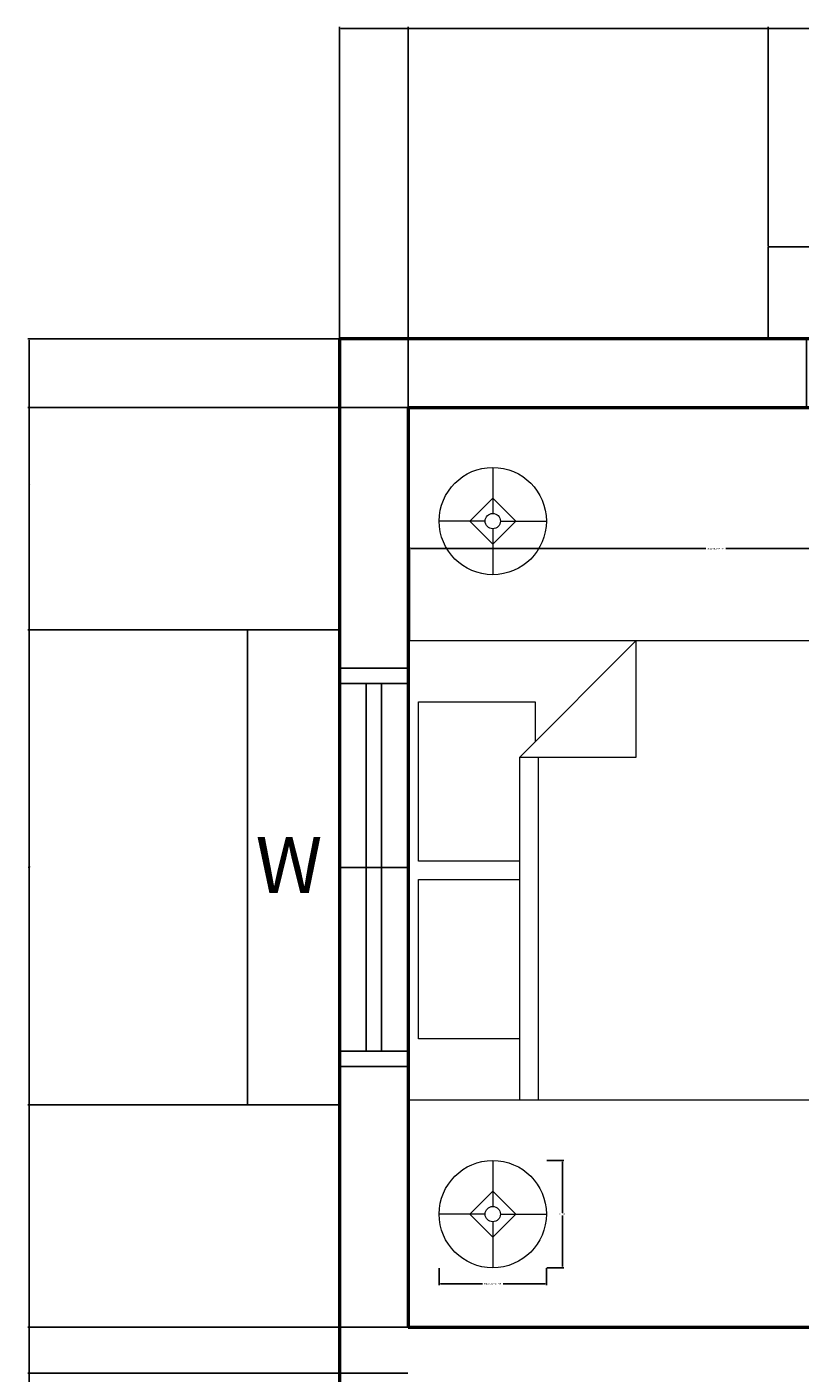
# Model space of a CAD drawing. Units: inches. Extents: x -73 to 1162, y -188 to 590.
# Tile 2 of 9: x -73 to 28, y 17 to 193. Entities that reach past the tile are written whole.
import ezdxf

# ---------------------------------------------------------------- set-up
doc = ezdxf.new("R2010")
doc.units = ezdxf.units.IN
doc.header["$MEASUREMENT"] = 0
for name, color, linetype, lineweight in [('A-ANNO-DIMS', 2, 'Continuous', 18), ('A-ANNO-TEXT', 7, 'Continuous', 25), ('A-FURN', 8, 'Continuous', 18), ('A-GLAZ', 4, 'Continuous', 25), ('A-WALL', 7, 'Continuous', 50)]:
    doc.layers.add(name, color=color, linetype=linetype, lineweight=lineweight)
doc.styles.get("Standard").update_dxf_attribs({"font": 'arial.ttf'})
doc.dimstyles.get("Standard").update_dxf_attribs({"dimtxt": 0.18, "dimasz": 0.18, "dimexe": 0.18, "dimexo": 0.0625, "dimgap": 0.09, "dimtad": 0, "dimtih": 1, "dimtoh": 1, "dimdec": 1, "dimzin": 0, "dimdsep": 46, "dimlunit": 4, "dimtxsty": 'Standard', "dimcen": 0.09, "dimadec": 0, "dimazin": 0, "dimtfac": 1, "dimtdec": 1, "dimtofl": 0, "dimtmove": 0, "dimatfit": 3, "dimfxl": 1, "dimtolj": 1, "dimtzin": 0, "dimarcsym": 0})

# ---------------------------------------------------------------- blocks, each defined once
blk = doc.blocks.new('Bed - Queen')
for p, q in [((0, -80.00003), (0, 0)), ((0, 0), (59.99999, 0)), ((59.99999, 0), (59.99999, -80.00003)), ((7.99999, -1.2), (28.79998, -1.2)), ((7.99999, -14.4), (7.99999, -1.2)), ((28.79998, -1.2), (28.79998, -14.4)), ((31.19999, -1.2), (51.99999, -1.2)), ((31.19999, -14.4), (31.19999, -1.2)), ((51.99999, -1.2), (51.99999, -16.4)), ((0, -14.4), (44.8, -14.4)), ((59.99999, -29.6), (44.8, -14.4)), ((44.8, -14.4), (44.8, -29.6)), ((44.8, -16.8), (0, -16.8)), ((51.99999, -16.4), (46.79936, -16.4)), ((44.8, -29.6), (59.99999, -29.6)), ((59.99999, -80.00003), (0, -80.00003))]:
    blk.add_line(p, q)
blk = doc.blocks.new('Lamp - Table')
for p, q in [((0, 7), (0, 1)), ((0, 3), (-3, 0)), ((3, 0), (0, 3)), ((-1, 0), (-7, 0)), ((-3, 0), (0, -3)), ((0, -3), (3, 0)), ((1, 0), (7, 0)), ((0, -1), (0, -7))]:
    blk.add_line(p, q)
for radius in [7, 1]:
    blk.add_circle((0, 0), radius)
blk = doc.blocks.new('WIN-W')
for p, q in [((9, 57), (9, 62)), ((9, 62), (21, 62)), ((21, 62), (21, 0)), ((0, 57), (9, 57)), ((0, 5), (9, 5)), ((9, 5), (9, 0)), ((9, 0), (21, 0))]:
    blk.add_line(p, q)
blk = doc.blocks.new('*D34')
at = {"layer": 'A-ANNO-DIMS', "color": 0, "lineweight": -2, "transparency": 16777216}
for p, q in [((-22.68, 112.85), (-22.68, 124.96)), ((-22.5, 124.78), (16.02, 124.78)), ((57.14, 124.78), (18.63, 124.78)), ((57.32, 112.85), (57.32, 124.96))]:
    blk.add_line(p, q, dxfattribs=at)
at = {"layer": 'A-ANNO-DIMS', "color": 0, "transparency": 16777216}
for points in [[(-22.5, 124.81), (-22.5, 124.75), (-22.68, 124.78)], [(57.14, 124.81), (57.14, 124.75), (57.32, 124.78)]]:
    blk.add_solid(points, dxfattribs=at)
at = {"layer": 'Defpoints', "color": 0, "transparency": 16777216}
for p in [(-22.68, 124.78), (-22.68, 112.78), (57.32, 112.78)]:
    blk.add_point(p, dxfattribs=at)
at = {"layer": 'A-ANNO-DIMS', "color": 0, "transparency": 16777216, "insert": (17.32, 124.78), "char_height": 0.18, "attachment_point": 5}
blk.add_mtext('\\A1;QUEEN BED 80 TYP.', dxfattribs=at)
blk = doc.blocks.new('*D36')
at = {"layer": 'A-ANNO-DIMS', "color": 0, "lineweight": -2, "transparency": 16777216}
for p, q in [((-18.79, 30.87), (-18.79, 28.65)), ((-4.79, 30.87), (-4.79, 28.65)), ((-18.61, 28.83), (-13.13, 28.83)), ((-4.97, 28.83), (-10.45, 28.83))]:
    blk.add_line(p, q, dxfattribs=at)
at = {"layer": 'A-ANNO-DIMS', "color": 0, "transparency": 16777216}
for points in [[(-18.61, 28.86), (-18.61, 28.8), (-18.79, 28.83)], [(-4.97, 28.86), (-4.97, 28.8), (-4.79, 28.83)]]:
    blk.add_solid(points, dxfattribs=at)
at = {"layer": 'Defpoints', "color": 0, "transparency": 16777216}
for p in [(-18.79, 30.93), (-4.79, 30.93), (-4.79, 28.83)]:
    blk.add_point(p, dxfattribs=at)
at = {"layer": 'A-ANNO-DIMS', "color": 0, "transparency": 16777216, "insert": (-11.79, 28.83), "char_height": 0.18, "attachment_point": 5}
blk.add_mtext('\\A1;TABLE LAMP 14 TYP.', dxfattribs=at)
blk = doc.blocks.new('*D37')
at = {"layer": 'A-ANNO-DIMS', "color": 0, "lineweight": -2, "transparency": 16777216}
for p, q in [((-4.73, 44.93), (-2.51, 44.93)), ((-2.69, 44.75), (-2.69, 38.11)), ((-2.69, 31.11), (-2.69, 37.75)), ((-4.73, 30.93), (-2.51, 30.93))]:
    blk.add_line(p, q, dxfattribs=at)
at = {"layer": 'A-ANNO-DIMS', "color": 0, "transparency": 16777216}
for points in [[(-2.72, 44.75), (-2.66, 44.75), (-2.69, 44.93)], [(-2.72, 31.11), (-2.66, 31.11), (-2.69, 30.93)]]:
    blk.add_solid(points, dxfattribs=at)
at = {"layer": 'Defpoints', "color": 0, "transparency": 16777216}
for p in [(-4.79, 44.93), (-2.69, 44.93), (-4.79, 30.93)]:
    blk.add_point(p, dxfattribs=at)
at = {"layer": 'A-ANNO-DIMS', "color": 0, "transparency": 16777216, "insert": (-2.69, 37.93), "char_height": 0.18, "attachment_point": 5}
blk.add_mtext('\\A1;14 TYP.', dxfattribs=at)
blk = doc.blocks.new('*D59')
at = {"layer": 'A-ANNO-DIMS', "color": 0, "lineweight": -2, "transparency": 16777216}
for p, q in [((-31.83, 152.25), (-31.83, 192.86)), ((-31.65, 192.68), (-4.05, 192.68)), ((23.99, 192.68), (-3.61, 192.68)), ((24.17, 164.25), (24.17, 192.86))]:
    blk.add_line(p, q, dxfattribs=at)
at = {"layer": 'A-ANNO-DIMS', "color": 0, "transparency": 16777216}
for points in [[(-31.65, 192.71), (-31.65, 192.65), (-31.83, 192.68)], [(23.99, 192.71), (23.99, 192.65), (24.17, 192.68)]]:
    blk.add_solid(points, dxfattribs=at)
at = {"layer": 'Defpoints', "color": 0, "transparency": 16777216}
for p in [(24.17, 192.68), (24.17, 164.18), (-31.83, 152.18)]:
    blk.add_point(p, dxfattribs=at)
at = {"layer": 'A-ANNO-DIMS', "color": 0, "transparency": 16777216, "insert": (-3.83, 192.68), "char_height": 0.18, "attachment_point": 5}
blk.add_mtext('\\A1;56', dxfattribs=at)
blk = doc.blocks.new('*D65')
at = {"layer": 'A-ANNO-DIMS', "color": 0, "lineweight": -2, "transparency": 16777216}
for p, q in [((-31.89, 152.18), (-72.51, 152.18)), ((-72.33, 152), (-72.33, 2.37)), ((-72.33, -147.64), (-72.33, 2)), ((-31.89, -147.82), (-72.51, -147.82))]:
    blk.add_line(p, q, dxfattribs=at)
at = {"layer": 'A-ANNO-DIMS', "color": 0, "transparency": 16777216}
for points in [[(-72.36, 152), (-72.3, 152), (-72.33, 152.18)], [(-72.36, -147.64), (-72.3, -147.64), (-72.33, -147.82)]]:
    blk.add_solid(points, dxfattribs=at)
at = {"layer": 'Defpoints', "color": 0, "transparency": 16777216}
for p in [(-31.83, 152.18), (-72.33, -147.82), (-31.83, -147.82)]:
    blk.add_point(p, dxfattribs=at)
at = {"layer": 'A-ANNO-DIMS', "color": 0, "transparency": 16777216, "insert": (-72.33, 2.18), "char_height": 0.18, "attachment_point": 5}
blk.add_mtext('\\A1;300', dxfattribs=at)
blk = doc.blocks.new('*D66')
at = {"layer": 'A-ANNO-DIMS', "color": 0, "lineweight": -2, "transparency": 16777216}
for p, q in [((-31.89, 152.18), (-72.51, 152.18)), ((-72.33, 152), (-72.33, 133.37)), ((-72.33, 114.36), (-72.33, 133)), ((-43.89, 114.18), (-72.51, 114.18))]:
    blk.add_line(p, q, dxfattribs=at)
at = {"layer": 'A-ANNO-DIMS', "color": 0, "transparency": 16777216}
for points in [[(-72.36, 152), (-72.3, 152), (-72.33, 152.18)], [(-72.36, 114.36), (-72.3, 114.36), (-72.33, 114.18)]]:
    blk.add_solid(points, dxfattribs=at)
at = {"layer": 'Defpoints', "color": 0, "transparency": 16777216}
for p in [(-31.83, 152.18), (-72.33, 114.18), (-43.83, 114.18)]:
    blk.add_point(p, dxfattribs=at)
at = {"layer": 'A-ANNO-DIMS', "color": 0, "transparency": 16777216, "insert": (-72.33, 133.18), "char_height": 0.18, "attachment_point": 5}
blk.add_mtext('\\A1;38', dxfattribs=at)
blk = doc.blocks.new('*D67')
at = {"layer": 'A-ANNO-DIMS', "color": 0, "lineweight": -2, "transparency": 16777216}
for p, q in [((-43.89, 52.18), (-72.51, 52.18)), ((-72.33, 52), (-72.33, 12.04)), ((-72.33, -28.3), (-72.33, 11.67)), ((-43.89, -28.48), (-72.51, -28.48))]:
    blk.add_line(p, q, dxfattribs=at)
at = {"layer": 'A-ANNO-DIMS', "color": 0, "transparency": 16777216}
for points in [[(-72.36, 52), (-72.3, 52), (-72.33, 52.18)], [(-72.36, -28.3), (-72.3, -28.3), (-72.33, -28.48)]]:
    blk.add_solid(points, dxfattribs=at)
at = {"layer": 'Defpoints', "color": 0, "transparency": 16777216}
for p in [(-43.83, 52.18), (-72.33, -28.48), (-43.83, -28.48)]:
    blk.add_point(p, dxfattribs=at)
at = {"layer": 'A-ANNO-DIMS', "color": 0, "transparency": 16777216, "insert": (-72.33, 11.85), "char_height": 0.18, "attachment_point": 5}
blk.add_mtext('\\A1;80.66', dxfattribs=at)
blk = doc.blocks.new('*D86')
at = {"layer": 'A-ANNO-DIMS', "color": 0, "lineweight": -2, "transparency": 16777216}
for p, q in [((-31.83, 152.25), (-31.83, 192.86)), ((-31.65, 192.68), (-27.48, 192.68)), ((-23.01, 192.68), (-27.18, 192.68)), ((-22.83, 143.25), (-22.83, 192.86))]:
    blk.add_line(p, q, dxfattribs=at)
at = {"layer": 'A-ANNO-DIMS', "color": 0, "transparency": 16777216}
for points in [[(-31.65, 192.71), (-31.65, 192.65), (-31.83, 192.68)], [(-23.01, 192.71), (-23.01, 192.65), (-22.83, 192.68)]]:
    blk.add_solid(points, dxfattribs=at)
at = {"layer": 'Defpoints', "color": 0, "transparency": 16777216}
for p in [(-22.83, 192.68), (-31.83, 152.18), (-22.83, 143.18)]:
    blk.add_point(p, dxfattribs=at)
at = {"layer": 'A-ANNO-DIMS', "color": 0, "transparency": 16777216, "insert": (-27.33, 192.68), "char_height": 0.18, "attachment_point": 5}
blk.add_mtext('\\A1;9', dxfattribs=at)
blk = doc.blocks.new('*D88')
at = {"layer": 'A-ANNO-DIMS', "color": 0, "lineweight": -2, "transparency": 16777216}
for p, q in [((-22.83, 143.25), (-22.83, 192.86)), ((-22.65, 192.68), (54.89, 192.68)), ((132.99, 192.68), (55.45, 192.68)), ((133.17, 143.25), (133.17, 192.86))]:
    blk.add_line(p, q, dxfattribs=at)
at = {"layer": 'A-ANNO-DIMS', "color": 0, "transparency": 16777216}
for points in [[(-22.65, 192.71), (-22.65, 192.65), (-22.83, 192.68)], [(132.99, 192.71), (132.99, 192.65), (133.17, 192.68)]]:
    blk.add_solid(points, dxfattribs=at)
at = {"layer": 'Defpoints', "color": 0, "transparency": 16777216}
for p in [(133.17, 192.68), (-22.83, 143.18), (133.17, 143.18)]:
    blk.add_point(p, dxfattribs=at)
at = {"layer": 'A-ANNO-DIMS', "color": 0, "transparency": 16777216, "insert": (55.17, 192.68), "char_height": 0.18, "attachment_point": 5}
blk.add_mtext('\\A1;156', dxfattribs=at)
blk = doc.blocks.new('*D92')
at = {"layer": 'A-ANNO-DIMS', "color": 0, "lineweight": -2, "transparency": 16777216}
for p, q in [((-22.89, 143.18), (-72.51, 143.18)), ((-72.33, 143), (-72.33, 83.37)), ((-72.33, 23.36), (-72.33, 83)), ((-22.89, 23.18), (-72.51, 23.18))]:
    blk.add_line(p, q, dxfattribs=at)
at = {"layer": 'A-ANNO-DIMS', "color": 0, "transparency": 16777216}
for points in [[(-72.36, 143), (-72.3, 143), (-72.33, 143.18)], [(-72.36, 23.36), (-72.3, 23.36), (-72.33, 23.18)]]:
    blk.add_solid(points, dxfattribs=at)
at = {"layer": 'Defpoints', "color": 0, "transparency": 16777216}
for p in [(-22.83, 143.18), (-72.33, 23.18), (-22.83, 23.18)]:
    blk.add_point(p, dxfattribs=at)
at = {"layer": 'A-ANNO-DIMS', "color": 0, "transparency": 16777216, "insert": (-72.33, 83.18), "char_height": 0.18, "attachment_point": 5}
blk.add_mtext('\\A1;120', dxfattribs=at)
blk = doc.blocks.new('*D98')
at = {"layer": 'A-ANNO-DIMS', "color": 0, "lineweight": -2, "transparency": 16777216}
for p, q in [((-22.89, 17.18), (-72.51, 17.18)), ((-72.33, 17), (-72.33, -60.63)), ((-72.33, -138.64), (-72.33, -61)), ((-22.89, -138.82), (-72.51, -138.82))]:
    blk.add_line(p, q, dxfattribs=at)
at = {"layer": 'A-ANNO-DIMS', "color": 0, "transparency": 16777216}
for points in [[(-72.36, 17), (-72.3, 17), (-72.33, 17.18)], [(-72.36, -138.64), (-72.3, -138.64), (-72.33, -138.82)]]:
    blk.add_solid(points, dxfattribs=at)
at = {"layer": 'Defpoints', "color": 0, "transparency": 16777216}
for p in [(-72.33, 17.18), (-22.83, 17.18), (-22.83, -138.82)]:
    blk.add_point(p, dxfattribs=at)
at = {"layer": 'A-ANNO-DIMS', "color": 0, "transparency": 16777216, "insert": (-72.33, -60.82), "char_height": 0.18, "attachment_point": 5}
blk.add_mtext('\\A1;156', dxfattribs=at)

msp = doc.modelspace()

# ---------------------------------------------------------------- linework, layer by layer
at = {"layer": 'A-GLAZ'}
for p, q in [((-22.83, 107.1844), (-31.83, 107.1844)), ((-28.33, 59.1844), (-28.33, 107.1844)), ((-26.33, 59.1844), (-26.33, 107.1844)), ((-22.83, 83.1844), (-31.83, 83.1844)), ((-22.83, 59.1844), (-31.83, 59.1844))]:
    msp.add_line(p, q, dxfattribs=at)
at = {"layer": 'A-WALL'}
for p, q in [((-31.83, 152.1844), (139.17, 152.1844)), ((-31.83, 152.1844), (-31.83, 23.1844)), ((-22.83, 143.1844), (133.17, 143.1844)), ((-22.83, 143.1844), (-22.83, 23.1844)), ((-31.83, 23.1844), (-31.83, -147.8156)), ((-22.83, 23.1844), (139.17, 23.1844))]:
    msp.add_line(p, q, dxfattribs=at)

# ---------------------------------------------------------------- block references
at = {"layer": 'A-FURN'}
for p in [(-11.7901, 128.374), (-11.7901, 37.9281)]:
    msp.add_blockref('Lamp - Table', p, dxfattribs=at)
at = {"layer": 'A-FURN', "rotation": 90}
msp.add_blockref('Bed - Queen', (-22.6767, 52.7839), dxfattribs=at)
at = {"layer": 'A-GLAZ'}
for p, rotation in [((86.1704, 143.1844), 89.99999999999999), ((-22.83, 114.1849), 180)]:
    msp.add_blockref('WIN-W', p, dxfattribs=dict(at, rotation=rotation))

# ---------------------------------------------------------------- texts
at = {"layer": 'A-ANNO-TEXT'}
msp.add_text('W', height=7.2829, dxfattribs=at).set_placement((-42.7697, 79.8501))

# ---------------------------------------------------------------- dimensions: what is measured, and where the dimension line sits
at = {"layer": 'A-ANNO-DIMS'}
for base, p1, p2, picture, middle in [((24.17, 192.6844), (-31.83, 152.1844), (24.17, 164.1844), '*D59', (-3.83, 192.6844)), ((-22.83, 192.6844), (-31.83, 152.1844), (-22.83, 143.1844), '*D86', (-27.33, 192.6844)), ((133.17, 192.6844), (-22.83, 143.1844), (133.17, 143.1844), '*D88', (55.17, 192.6844))]:
    dim = msp.add_linear_dim(base=base, p1=p1, p2=p2, dimstyle='Standard', override={"dimdec": 0, "dimlfac": 1, "dimrnd": 0, "dimzin": 0, "dimdsep": 46, "dimlunit": 2}, dxfattribs=at)
    dim.commit()
    dim.dimension.update_dxf_attribs({"geometry": picture, "text_midpoint": middle})
for base, p1, p2, override, picture, middle in [((-72.33, -147.8156), (-31.83, 152.1844), (-31.83, -147.8156), {"dimdec": 0, "dimlfac": 1, "dimrnd": 0, "dimzin": 0, "dimdsep": 46, "dimlunit": 2}, '*D65', (-72.33, 2.1844)), ((-72.33, 114.1844), (-31.83, 152.1844), (-43.83, 114.1844), {"dimdec": 0, "dimlfac": 1, "dimrnd": 0, "dimzin": 0, "dimdsep": 46, "dimlunit": 2}, '*D66', (-72.33, 133.1844)), ((-72.33, 23.1844), (-22.83, 143.1844), (-22.83, 23.1844), {"dimdec": 0, "dimlfac": 1, "dimrnd": 0, "dimzin": 0, "dimdsep": 46, "dimlunit": 2}, '*D92', (-72.33, 83.1844)), ((-72.33, -28.4767), (-43.83, 52.1844), (-43.83, -28.4767), {"dimdec": 2, "dimlfac": 1, "dimrnd": 0, "dimzin": 0, "dimdsep": 46, "dimlunit": 2}, '*D67', (-72.33, 11.8538)), ((-72.33, 17.1844), (-22.83, -138.8156), (-22.83, 17.1844), {"dimdec": 0, "dimlfac": 1, "dimrnd": 0, "dimzin": 0, "dimdsep": 46, "dimlunit": 2}, '*D98', (-72.33, -60.8156))]:
    dim = msp.add_linear_dim(base=base, p1=p1, p2=p2, angle=90, dimstyle='Standard', override=override, dxfattribs=at)
    dim.commit()
    dim.dimension.update_dxf_attribs({"geometry": picture, "text_midpoint": middle})
for base, p1, p2, angle, text, picture, middle in [((-22.6767, 124.7839), (57.3233, 112.7839), (-22.6767, 112.7839), 180, 'QUEEN BED <> TYP.', '*D34', (17.3233, 124.7839)), ((-2.6901, 44.9281), (-4.7901, 30.9281), (-4.7901, 44.9281), 90, '<> TYP.', '*D37', (-2.6901, 37.9281))]:
    dim = msp.add_linear_dim(base=base, p1=p1, p2=p2, angle=angle, text=text, dimstyle='Standard', override={"dimdec": 0, "dimrnd": 0, "dimzin": 0, "dimlunit": 2}, dxfattribs=at)
    dim.commit()
    dim.dimension.update_dxf_attribs({"geometry": picture, "text_midpoint": middle})
dim = msp.add_linear_dim(base=(-4.7901, 28.8281), p1=(-18.7901, 30.9281), p2=(-4.7901, 30.9281), text='TABLE LAMP <> TYP.', dimstyle='Standard', override={"dimdec": 0, "dimrnd": 0, "dimzin": 0, "dimlunit": 2}, dxfattribs=at)
dim.commit()
dim.dimension.update_dxf_attribs({"geometry": '*D36', "text_midpoint": (-11.7901, 28.8281)})

doc.saveas('drawing.dxf')
